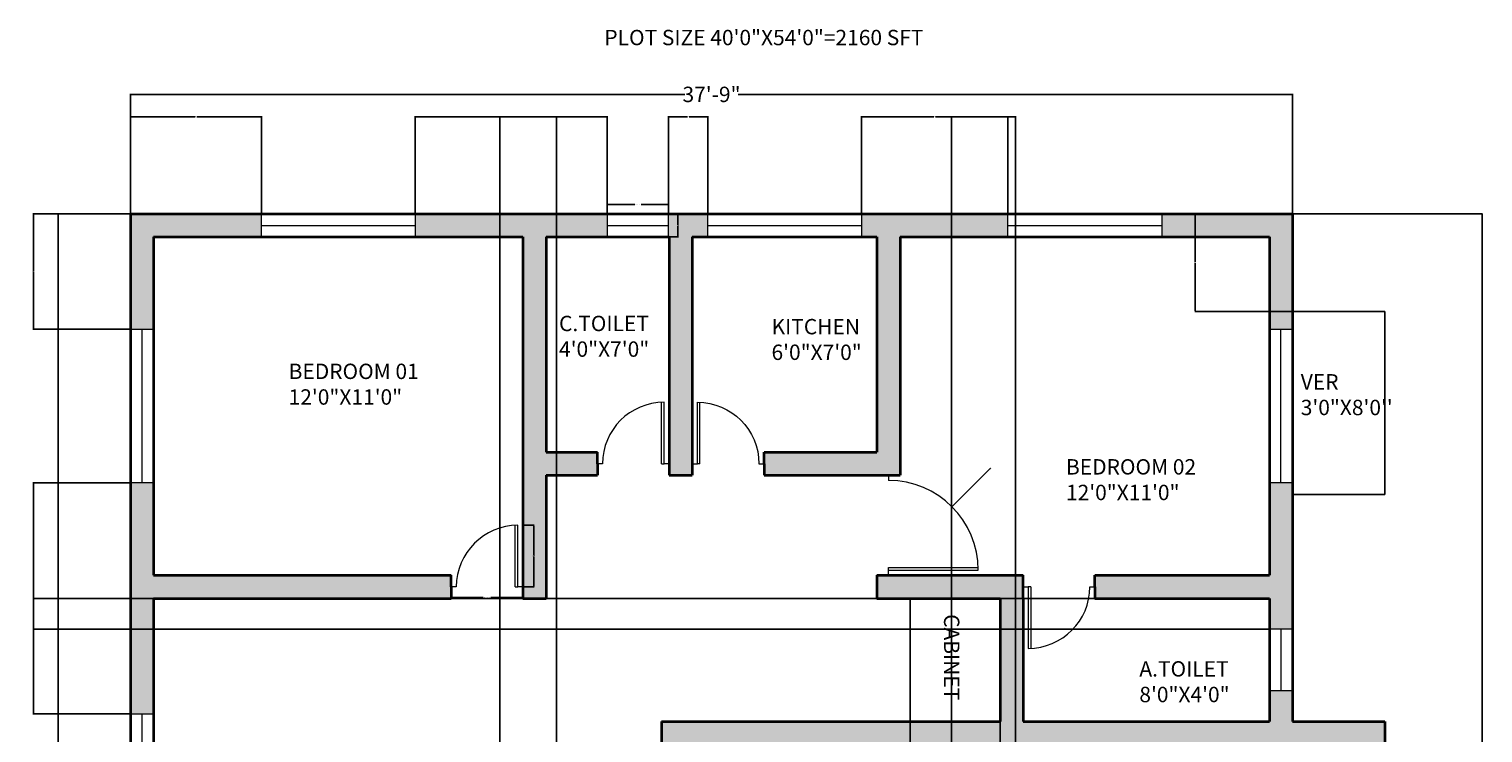
# Model space of a CAD drawing. Units: inches. Extents: x -17 to 550, y -704 to 87.
# Tile 2 of 2: x -17 to 550, y -187 to 87. Entities that reach past the tile are written whole.
import ezdxf

# ---------------------------------------------------------------- set-up
doc = ezdxf.new("R2010")
doc.units = ezdxf.units.IN
doc.header["$MEASUREMENT"] = 0
for name, color, linetype, lineweight in [('A-ANNO-DIMS', 2, 'Continuous', 18), ('A-ANNO-TEXT', 7, 'Continuous', 18), ('A-AREA-IDEN', 7, 'Continuous', 18), ('A-DOOR', 3, 'Continuous', 18), ('A-FLOR-CASE', 8, 'Continuous', 18), ('A-FLOR-OTLN', 7, 'Continuous', 25), ('A-GLAZ', 4, 'Continuous', 18), ('A-WALL', 7, 'Continuous', 35), ('A-WALL-PATT', 252, 'Continuous', 13)]:
    doc.layers.add(name, color=color, linetype=linetype, lineweight=lineweight)
doc.styles.get("Standard").update_dxf_attribs({"font": 'arial.ttf'})
doc.dimstyles.get("Standard").update_dxf_attribs({"dimtxt": 0.18, "dimasz": 0.18, "dimexe": 0.18, "dimexo": 0.0625, "dimgap": 0.09, "dimtad": 0, "dimtih": 1, "dimtoh": 1, "dimdec": 0, "dimzin": 0, "dimdsep": 46, "dimlunit": 3, "dimtxsty": 'Standard', "dimcen": 0.09, "dimadec": 0, "dimazin": 0, "dimtfac": 1, "dimtdec": 0, "dimtofl": 0, "dimtmove": 0, "dimatfit": 3, "dimfxl": 1, "dimtolj": 1, "dimtzin": 0, "dimarcsym": 0})

# ---------------------------------------------------------------- blocks, each defined once
blk = doc.blocks.new('*D1')
at = {"layer": 'A-ANNO-DIMS', "color": 0, "lineweight": -2, "transparency": 16777216}
for p, q in [((22.74, 15.39), (22.74, 62.1)), ((22.92, 61.92), (238.85, 61.92)), ((475.56, 61.92), (259.64, 61.92)), ((475.74, 15.39), (475.74, 62.1))]:
    blk.add_line(p, q, dxfattribs=at)
at = {"layer": 'A-ANNO-DIMS', "color": 0, "transparency": 16777216}
for points in [[(22.92, 61.95), (22.92, 61.89), (22.74, 61.92)], [(475.56, 61.95), (475.56, 61.89), (475.74, 61.92)]]:
    blk.add_solid(points, dxfattribs=at)
at = {"layer": 'Defpoints', "color": 0, "transparency": 16777216}
for p in [(475.74, 61.92), (22.74, 15.33), (475.74, 15.33)]:
    blk.add_point(p, dxfattribs=at)
at = {"layer": 'A-ANNO-DIMS', "color": 0, "transparency": 16777216, "insert": (249.24, 61.92), "char_height": 6, "attachment_point": 5}
blk.add_mtext('\\A1;37\'-9"', dxfattribs=at)
blk = doc.blocks.new('*D2')
at = {"layer": 'A-ANNO-DIMS', "color": 0, "lineweight": -2, "transparency": 16777216}
for p, q in [((22.68, 15.33), (-5.69, 15.33)), ((-5.51, 15.15), (-5.51, -322.02)), ((-5.51, -665.49), (-5.51, -328.33)), ((22.68, -665.67), (-5.69, -665.67))]:
    blk.add_line(p, q, dxfattribs=at)
at = {"layer": 'A-ANNO-DIMS', "color": 0, "transparency": 16777216}
for points in [[(-5.54, 15.15), (-5.48, 15.15), (-5.51, 15.33)], [(-5.54, -665.49), (-5.48, -665.49), (-5.51, -665.67)]]:
    blk.add_solid(points, dxfattribs=at)
at = {"layer": 'Defpoints', "color": 0, "transparency": 16777216}
for p in [(22.74, 15.33), (-5.51, -665.67), (22.74, -665.67)]:
    blk.add_point(p, dxfattribs=at)
at = {"layer": 'A-ANNO-DIMS', "color": 0, "transparency": 16777216, "insert": (-5.51, -325.17), "char_height": 6, "attachment_point": 5}
blk.add_mtext('\\A1;56\'-9"', dxfattribs=at)
blk = doc.blocks.new('WIN-60IN')
for p, q in [((0, 9), (60, 9)), ((0, 0), (0, 9)), ((60, 9), (60, 0)), ((0, 4.5), (60, 4.5)), ((60, 0), (0, 0))]:
    blk.add_line(p, q)
blk = doc.blocks.new('WIN-24IN')
for p, q in [((0, 24), (0, 0)), ((9, 24), (0, 24)), ((4.5, 24), (4.5, 0)), ((9, 0), (9, 24)), ((0, 0), (9, 0))]:
    blk.add_line(p, q)
blk = doc.blocks.new('DOOR-SWING-24IN')
for p, q in [((25, 0), (25, 24)), ((26, 0), (26, 24)), ((2, 0), (0, 0)), ((25, 0), (26, 0)), ((28, 0), (26, 0))]:
    blk.add_line(p, q)
blk.add_arc((26, 0), 24, 90, 180)
blk = doc.blocks.new('*D8')
at = {"layer": 'A-ANNO-DIMS', "color": 0, "lineweight": -2, "transparency": 16777216}
for p, q in [((147.74, -130.24), (147.74, -134.55)), ((175.74, -130.24), (175.74, -134.55)), ((147.92, -134.37), (160.23, -134.37)), ((175.56, -134.37), (163.25, -134.37))]:
    blk.add_line(p, q, dxfattribs=at)
at = {"layer": 'A-ANNO-DIMS', "color": 0, "transparency": 16777216}
for points in [[(147.92, -134.34), (147.92, -134.4), (147.74, -134.37)], [(175.56, -134.34), (175.56, -134.4), (175.74, -134.37)]]:
    blk.add_solid(points, dxfattribs=at)
at = {"layer": 'Defpoints', "color": 0, "transparency": 16777216}
for p in [(147.74, -130.17), (175.74, -130.17), (175.74, -134.37)]:
    blk.add_point(p, dxfattribs=at)
at = {"layer": 'A-ANNO-DIMS', "color": 0, "transparency": 16777216, "insert": (161.74, -134.37), "char_height": 0.18, "attachment_point": 5}
blk.add_mtext('\\A1;SWING DOOR 2\'-4" TYP.', dxfattribs=at)
blk = doc.blocks.new('*D9')
at = {"layer": 'A-ANNO-DIMS', "color": 0, "lineweight": -2, "transparency": 16777216}
for p, q in [((175.81, -106.17), (180.12, -106.17)), ((179.94, -106.35), (179.94, -117.99)), ((179.94, -129.99), (179.94, -118.36)), ((175.81, -130.17), (180.12, -130.17))]:
    blk.add_line(p, q, dxfattribs=at)
at = {"layer": 'A-ANNO-DIMS', "color": 0, "transparency": 16777216}
for points in [[(179.91, -106.35), (179.97, -106.35), (179.94, -106.17)], [(179.91, -129.99), (179.97, -129.99), (179.94, -130.17)]]:
    blk.add_solid(points, dxfattribs=at)
at = {"layer": 'Defpoints', "color": 0, "transparency": 16777216}
for p in [(175.74, -106.17), (179.94, -106.17), (175.74, -130.17)]:
    blk.add_point(p, dxfattribs=at)
at = {"layer": 'A-ANNO-DIMS', "color": 0, "transparency": 16777216, "insert": (179.94, -118.17), "char_height": 0.18, "attachment_point": 5}
blk.add_mtext('\\A1;2\'-0" TYP.', dxfattribs=at)
blk = doc.blocks.new('*D12')
at = {"layer": 'A-ANNO-DIMS', "color": 0, "lineweight": -2, "transparency": 16777216}
for p, q in [((208.53, 15.39), (208.53, 19.11)), ((208.71, 18.93), (219.31, 18.93)), ((232.35, 18.93), (221.76, 18.93)), ((232.53, 15.39), (232.53, 19.11))]:
    blk.add_line(p, q, dxfattribs=at)
at = {"layer": 'A-ANNO-DIMS', "color": 0, "transparency": 16777216}
for points in [[(208.71, 18.96), (208.71, 18.9), (208.53, 18.93)], [(232.35, 18.96), (232.35, 18.9), (232.53, 18.93)]]:
    blk.add_solid(points, dxfattribs=at)
at = {"layer": 'Defpoints', "color": 0, "transparency": 16777216}
for p in [(208.53, 18.93), (208.53, 15.33), (232.53, 15.33)]:
    blk.add_point(p, dxfattribs=at)
at = {"layer": 'A-ANNO-DIMS', "color": 0, "transparency": 16777216, "insert": (220.53, 18.93), "char_height": 0.18, "attachment_point": 5}
blk.add_mtext('\\A1;WINDOW 2\'-0" TYP.', dxfattribs=at)
blk = doc.blocks.new('*D13')
at = {"layer": 'A-ANNO-DIMS', "color": 0, "lineweight": -2, "transparency": 16777216}
for p, q in [((232.6, 15.33), (236.31, 15.33)), ((236.13, 15.15), (236.13, 11.01)), ((232.6, 6.33), (236.31, 6.33)), ((236.13, 6.51), (236.13, 10.64))]:
    blk.add_line(p, q, dxfattribs=at)
at = {"layer": 'A-ANNO-DIMS', "color": 0, "transparency": 16777216}
for points in [[(236.1, 15.15), (236.16, 15.15), (236.13, 15.33)], [(236.1, 6.51), (236.16, 6.51), (236.13, 6.33)]]:
    blk.add_solid(points, dxfattribs=at)
at = {"layer": 'Defpoints', "color": 0, "transparency": 16777216}
for p in [(232.53, 15.33), (236.13, 15.33), (232.53, 6.33)]:
    blk.add_point(p, dxfattribs=at)
at = {"layer": 'A-ANNO-DIMS', "color": 0, "transparency": 16777216, "insert": (236.13, 10.83), "char_height": 0.18, "attachment_point": 5}
blk.add_mtext('\\A1;0\'-9" TYP.', dxfattribs=at)
blk = doc.blocks.new('*D23')
at = {"layer": 'A-ANNO-DIMS', "color": 0, "lineweight": -2, "transparency": 16777216}
for p, q in [((22.74, 15.39), (22.74, 53.41)), ((22.92, 53.23), (47.91, 53.23)), ((73.56, 53.23), (48.58, 53.23)), ((73.74, 15.39), (73.74, 53.41))]:
    blk.add_line(p, q, dxfattribs=at)
at = {"layer": 'A-ANNO-DIMS', "color": 0, "transparency": 16777216}
for points in [[(22.92, 53.26), (22.92, 53.2), (22.74, 53.23)], [(73.56, 53.26), (73.56, 53.2), (73.74, 53.23)]]:
    blk.add_solid(points, dxfattribs=at)
at = {"layer": 'Defpoints', "color": 0, "transparency": 16777216}
for p in [(73.74, 53.23), (22.74, 15.33), (73.74, 15.33)]:
    blk.add_point(p, dxfattribs=at)
at = {"layer": 'A-ANNO-DIMS', "color": 0, "transparency": 16777216, "insert": (48.24, 53.23), "char_height": 0.18, "attachment_point": 5}
blk.add_mtext('\\A1;4\'-3"', dxfattribs=at)
blk = doc.blocks.new('*D24')
at = {"layer": 'A-ANNO-DIMS', "color": 0, "lineweight": -2, "transparency": 16777216}
for p, q in [((133.74, 15.39), (133.74, 53.41)), ((133.92, 53.23), (170.81, 53.23)), ((208.35, 53.23), (171.47, 53.23)), ((208.53, 15.39), (208.53, 53.41))]:
    blk.add_line(p, q, dxfattribs=at)
at = {"layer": 'A-ANNO-DIMS', "color": 0, "transparency": 16777216}
for points in [[(133.92, 53.26), (133.92, 53.2), (133.74, 53.23)], [(208.35, 53.26), (208.35, 53.2), (208.53, 53.23)]]:
    blk.add_solid(points, dxfattribs=at)
at = {"layer": 'Defpoints', "color": 0, "transparency": 16777216}
for p in [(208.53, 53.23), (133.74, 15.33), (208.53, 15.33)]:
    blk.add_point(p, dxfattribs=at)
at = {"layer": 'A-ANNO-DIMS', "color": 0, "transparency": 16777216, "insert": (171.14, 53.23), "char_height": 0.18, "attachment_point": 5}
blk.add_mtext('\\A1;6\'-3"', dxfattribs=at)
blk = doc.blocks.new('*D25')
at = {"layer": 'A-ANNO-DIMS', "color": 0, "lineweight": -2, "transparency": 16777216}
for p, q in [((232.53, 15.39), (232.53, 53.41)), ((232.71, 53.23), (239.82, 53.23)), ((247.56, 53.23), (240.46, 53.23)), ((247.74, 15.39), (247.74, 53.41))]:
    blk.add_line(p, q, dxfattribs=at)
at = {"layer": 'A-ANNO-DIMS', "color": 0, "transparency": 16777216}
for points in [[(232.71, 53.26), (232.71, 53.2), (232.53, 53.23)], [(247.56, 53.26), (247.56, 53.2), (247.74, 53.23)]]:
    blk.add_solid(points, dxfattribs=at)
at = {"layer": 'Defpoints', "color": 0, "transparency": 16777216}
for p in [(247.74, 53.23), (232.53, 15.33), (247.74, 15.33)]:
    blk.add_point(p, dxfattribs=at)
at = {"layer": 'A-ANNO-DIMS', "color": 0, "transparency": 16777216, "insert": (240.14, 53.23), "char_height": 0.18, "attachment_point": 5}
blk.add_mtext('\\A1;1\'-3"', dxfattribs=at)
blk = doc.blocks.new('*D26')
at = {"layer": 'A-ANNO-DIMS', "color": 0, "lineweight": -2, "transparency": 16777216}
for p, q in [((307.74, 15.39), (307.74, 53.41)), ((307.92, 53.23), (335.91, 53.23)), ((364.56, 53.23), (336.58, 53.23)), ((364.74, 15.39), (364.74, 53.41))]:
    blk.add_line(p, q, dxfattribs=at)
at = {"layer": 'A-ANNO-DIMS', "color": 0, "transparency": 16777216}
for points in [[(307.92, 53.26), (307.92, 53.2), (307.74, 53.23)], [(364.56, 53.26), (364.56, 53.2), (364.74, 53.23)]]:
    blk.add_solid(points, dxfattribs=at)
at = {"layer": 'Defpoints', "color": 0, "transparency": 16777216}
for p in [(364.74, 53.23), (307.74, 15.33), (364.74, 15.33)]:
    blk.add_point(p, dxfattribs=at)
at = {"layer": 'A-ANNO-DIMS', "color": 0, "transparency": 16777216, "insert": (336.24, 53.23), "char_height": 0.18, "attachment_point": 5}
blk.add_mtext('\\A1;4\'-9"', dxfattribs=at)
blk = doc.blocks.new('*D27')
at = {"layer": 'A-ANNO-DIMS', "color": 0, "lineweight": -2, "transparency": 16777216}
for p, q in [((22.68, 15.33), (-15.34, 15.33)), ((-15.16, 15.15), (-15.16, -6.99)), ((-15.16, -29.49), (-15.16, -7.36)), ((22.68, -29.67), (-15.34, -29.67))]:
    blk.add_line(p, q, dxfattribs=at)
at = {"layer": 'A-ANNO-DIMS', "color": 0, "transparency": 16777216}
for points in [[(-15.19, 15.15), (-15.13, 15.15), (-15.16, 15.33)], [(-15.19, -29.49), (-15.13, -29.49), (-15.16, -29.67)]]:
    blk.add_solid(points, dxfattribs=at)
at = {"layer": 'Defpoints', "color": 0, "transparency": 16777216}
for p in [(-15.16, 15.33), (22.74, 15.33), (22.74, -29.67)]:
    blk.add_point(p, dxfattribs=at)
at = {"layer": 'A-ANNO-DIMS', "color": 0, "transparency": 16777216, "insert": (-15.16, -7.17), "char_height": 0.18, "attachment_point": 5}
blk.add_mtext('\\A1;3\'-9"', dxfattribs=at)
blk = doc.blocks.new('*D28')
at = {"layer": 'A-ANNO-DIMS', "color": 0, "lineweight": -2, "transparency": 16777216}
for p, q in [((22.68, -89.67), (-15.34, -89.67)), ((-15.16, -89.85), (-15.16, -134.49)), ((-15.16, -179.49), (-15.16, -134.86)), ((22.68, -179.67), (-15.34, -179.67))]:
    blk.add_line(p, q, dxfattribs=at)
at = {"layer": 'A-ANNO-DIMS', "color": 0, "transparency": 16777216}
for points in [[(-15.19, -89.85), (-15.13, -89.85), (-15.16, -89.67)], [(-15.19, -179.49), (-15.13, -179.49), (-15.16, -179.67)]]:
    blk.add_solid(points, dxfattribs=at)
at = {"layer": 'Defpoints', "color": 0, "transparency": 16777216}
for p in [(-15.16, -89.67), (22.74, -89.67), (22.74, -179.67)]:
    blk.add_point(p, dxfattribs=at)
at = {"layer": 'A-ANNO-DIMS', "color": 0, "transparency": 16777216, "insert": (-15.16, -134.67), "char_height": 0.18, "attachment_point": 5}
blk.add_mtext('\\A1;7\'-6"', dxfattribs=at)
blk = doc.blocks.new('*D32')
at = {"layer": 'A-ANNO-DIMS', "color": 0, "lineweight": -2, "transparency": 16777216}
for p, q in [((326.67, -134.74), (326.67, -703.75)), ((361.74, -134.74), (361.74, -703.75)), ((326.85, -703.57), (343.81, -703.57)), ((361.56, -703.57), (344.61, -703.57))]:
    blk.add_line(p, q, dxfattribs=at)
at = {"layer": 'A-ANNO-DIMS', "color": 0, "transparency": 16777216}
for points in [[(326.85, -703.54), (326.85, -703.6), (326.67, -703.57)], [(361.56, -703.54), (361.56, -703.6), (361.74, -703.57)]]:
    blk.add_solid(points, dxfattribs=at)
at = {"layer": 'Defpoints', "color": 0, "transparency": 16777216}
for p in [(326.67, -134.67), (361.74, -134.67), (361.74, -703.57)]:
    blk.add_point(p, dxfattribs=at)
at = {"layer": 'A-ANNO-DIMS', "color": 0, "transparency": 16777216, "insert": (344.21, -703.57), "char_height": 0.18, "attachment_point": 5}
blk.add_mtext('\\A1;2\'-11"', dxfattribs=at)
blk = doc.blocks.new('*D33')
at = {"layer": 'A-ANNO-DIMS', "color": 0, "lineweight": -2, "transparency": 16777216}
for p, q in [((166.74, -632.61), (166.74, 53.41)), ((166.92, 53.23), (177.41, 53.23)), ((188.68, 53.23), (178.19, 53.23)), ((188.86, -632.61), (188.86, 53.41))]:
    blk.add_line(p, q, dxfattribs=at)
at = {"layer": 'A-ANNO-DIMS', "color": 0, "transparency": 16777216}
for points in [[(166.92, 53.26), (166.92, 53.2), (166.74, 53.23)], [(188.68, 53.26), (188.68, 53.2), (188.86, 53.23)]]:
    blk.add_solid(points, dxfattribs=at)
at = {"layer": 'Defpoints', "color": 0, "transparency": 16777216}
for p in [(188.86, 53.23), (166.74, -632.67), (188.86, -632.67)]:
    blk.add_point(p, dxfattribs=at)
at = {"layer": 'A-ANNO-DIMS', "color": 0, "transparency": 16777216, "insert": (177.8, 53.23), "char_height": 0.18, "attachment_point": 5}
blk.add_mtext('\\A1;1\'-10"', dxfattribs=at)
blk = doc.blocks.new('*D34')
at = {"layer": 'A-ANNO-DIMS', "color": 0, "lineweight": -2, "transparency": 16777216}
for p, q in [((342.82, -632.61), (342.82, 53.41)), ((343, 53.23), (354.95, 53.23)), ((367.56, 53.23), (355.61, 53.23)), ((367.74, -632.61), (367.74, 53.41))]:
    blk.add_line(p, q, dxfattribs=at)
at = {"layer": 'A-ANNO-DIMS', "color": 0, "transparency": 16777216}
for points in [[(343, 53.26), (343, 53.2), (342.82, 53.23)], [(367.56, 53.26), (367.56, 53.2), (367.74, 53.23)]]:
    blk.add_solid(points, dxfattribs=at)
at = {"layer": 'Defpoints', "color": 0, "transparency": 16777216}
for p in [(367.74, 53.23), (342.82, -632.67), (367.74, -632.67)]:
    blk.add_point(p, dxfattribs=at)
at = {"layer": 'A-ANNO-DIMS', "color": 0, "transparency": 16777216, "insert": (355.28, 53.23), "char_height": 0.18, "attachment_point": 5}
blk.add_mtext('\\A1;2\'-1"', dxfattribs=at)
blk = doc.blocks.new('*D39')
at = {"layer": 'A-ANNO-DIMS', "color": 0, "lineweight": -2, "transparency": 16777216}
for p, q in [((466.68, -134.67), (-15.34, -134.67)), ((-15.16, -134.85), (-15.16, -140.49)), ((-15.16, -146.49), (-15.16, -140.86)), ((466.68, -146.67), (-15.34, -146.67))]:
    blk.add_line(p, q, dxfattribs=at)
at = {"layer": 'A-ANNO-DIMS', "color": 0, "transparency": 16777216}
for points in [[(-15.19, -134.85), (-15.13, -134.85), (-15.16, -134.67)], [(-15.19, -146.49), (-15.13, -146.49), (-15.16, -146.67)]]:
    blk.add_solid(points, dxfattribs=at)
at = {"layer": 'Defpoints', "color": 0, "transparency": 16777216}
for p in [(466.74, -134.67), (-15.16, -146.67), (466.74, -146.67)]:
    blk.add_point(p, dxfattribs=at)
at = {"layer": 'A-ANNO-DIMS', "color": 0, "transparency": 16777216, "insert": (-15.16, -140.67), "char_height": 0.18, "attachment_point": 5}
blk.add_mtext('\\A1;1\'-0"', dxfattribs=at)
blk = doc.blocks.new('*D40')
at = {"layer": 'A-ANNO-DIMS', "color": 0, "lineweight": -2, "transparency": 16777216}
for p, q in [((475.68, 15.33), (437.66, 15.33)), ((437.84, 15.15), (437.84, -3.51)), ((437.84, -22.53), (437.84, -3.87)), ((475.68, -22.71), (437.66, -22.71))]:
    blk.add_line(p, q, dxfattribs=at)
at = {"layer": 'A-ANNO-DIMS', "color": 0, "transparency": 16777216}
for points in [[(437.81, 15.15), (437.87, 15.15), (437.84, 15.33)], [(437.81, -22.53), (437.87, -22.53), (437.84, -22.71)]]:
    blk.add_solid(points, dxfattribs=at)
at = {"layer": 'Defpoints', "color": 0, "transparency": 16777216}
for p in [(437.84, 15.33), (475.74, 15.33), (475.74, -22.71)]:
    blk.add_point(p, dxfattribs=at)
at = {"layer": 'A-ANNO-DIMS', "color": 0, "transparency": 16777216, "insert": (437.84, -3.69), "char_height": 0.18, "attachment_point": 5}
blk.add_mtext('\\A1;3\'-2"', dxfattribs=at)
blk = doc.blocks.new('*D41')
at = {"layer": 'A-ANNO-DIMS', "color": 0, "lineweight": -2, "transparency": 16777216}
for p, q in [((475.81, 15.33), (549.82, 15.33)), ((549.64, 15.15), (549.64, -324.99)), ((549.64, -665.49), (549.64, -325.36)), ((511.81, -665.67), (549.82, -665.67))]:
    blk.add_line(p, q, dxfattribs=at)
at = {"layer": 'A-ANNO-DIMS', "color": 0, "transparency": 16777216}
for points in [[(549.61, 15.15), (549.67, 15.15), (549.64, 15.33)], [(549.61, -665.49), (549.67, -665.49), (549.64, -665.67)]]:
    blk.add_solid(points, dxfattribs=at)
at = {"layer": 'Defpoints', "color": 0, "transparency": 16777216}
for p in [(475.74, 15.33), (549.64, 15.33), (511.74, -665.67)]:
    blk.add_point(p, dxfattribs=at)
at = {"layer": 'A-ANNO-DIMS', "color": 0, "transparency": 16777216, "insert": (549.64, -325.17), "char_height": 0.18, "attachment_point": 5}
blk.add_mtext('\\A1;56\'-9"', dxfattribs=at)
blk = doc.blocks.new('*D42')
at = {"layer": 'A-ANNO-DIMS', "color": 0, "lineweight": -2, "transparency": 16777216}
for p, q in [((357.84, -84.08), (343.12, -98.8)), ((358.02, -84.08), (357.84, -84.08)), ((318.15, -123.67), (318.33, -123.67)), ((318.24, -123.76), (318.24, -123.58))]:
    blk.add_line(p, q, dxfattribs=at)
at = {"layer": 'A-ANNO-DIMS', "color": 0, "transparency": 16777216}
blk.add_solid([(343.1, -98.78), (343.14, -98.82), (342.99, -98.93)], dxfattribs=at)
at = {"layer": 'Defpoints', "color": 0, "transparency": 16777216}
for p in [(342.99, -98.93), (318.24, -123.67)]:
    blk.add_point(p, dxfattribs=at)
at = {"layer": 'A-ANNO-DIMS', "color": 0, "transparency": 16777216, "insert": (358.51, -84.08), "char_height": 0.18, "attachment_point": 5}
blk.add_mtext('\\A1;R2\'-11"', dxfattribs=at)

msp = doc.modelspace()

# ---------------------------------------------------------------- hatches: boundary and pattern name
at = {"layer": 'A-WALL-PATT'}
h = msp.add_hatch(color=256, dxfattribs=at)
h.dxf.hatch_style = 1
h.paths.add_polyline_path([(322.74, 6.33), (364.74, 6.33), (364.74, 15.33), (307.74, 15.33), (307.74, 6.33), (313.74, 6.33), (313.74, -77.67), (269.74, -77.67), (269.74, -82.17), (269.74, -86.67), (322.74, -86.67)])
h.paths.add_polyline_path([(475.74, 15.33), (424.74, 15.33), (424.74, 6.33), (466.74, 6.33), (466.74, -29.67), (475.74, -29.67)])
h.paths.add_polyline_path([(475.74, -89.67), (466.74, -89.67), (466.74, -125.67), (398.74, -125.67), (398.74, -130.17), (398.74, -134.67), (466.74, -134.67), (466.74, -146.67), (475.74, -146.67)])
h.paths.add_polyline_path([(511.74, -182.67), (475.74, -182.67), (475.74, -170.67), (466.74, -170.67), (466.74, -182.67), (370.74, -182.67), (370.74, -134.67), (370.74, -125.67), (313.74, -125.67), (313.74, -134.67), (361.74, -134.67), (361.74, -182.67), (229.74, -182.67), (229.74, -194.67), (238.74, -194.67), (238.74, -191.67), (502.74, -191.67), (502.74, -208.17), (511.74, -208.17)])
h.paths.add_polyline_path([(184.74, -86.67), (204.74, -86.67), (204.74, -82.17), (204.74, -77.67), (184.74, -77.67), (184.74, 6.33), (208.53, 6.33), (208.53, 15.33), (133.74, 15.33), (133.74, 6.33), (175.74, 6.33), (175.74, -134.67), (184.74, -134.67)])
h.paths.add_polyline_path([(241.74, 6.33), (247.74, 6.33), (247.74, 15.33), (232.53, 15.33), (232.53, 6.33), (232.74, 6.33), (232.74, -86.67), (241.74, -86.67)])
h.paths.add_polyline_path([(147.74, -125.67), (31.74, -125.67), (31.74, -89.67), (22.74, -89.67), (22.74, -179.67), (31.74, -179.67), (31.74, -134.67), (147.74, -134.67), (147.74, -130.17)])
h.paths.add_polyline_path([(31.74, 6.33), (73.74, 6.33), (73.74, 15.33), (22.74, 15.33), (22.74, -29.67), (31.74, -29.67)])
h.paths.add_polyline_path([(238.74, -284.67), (238.74, -222.67), (234.24, -222.67), (229.74, -222.67), (229.74, -284.67), (31.74, -284.67), (31.74, -239.67), (22.74, -239.67), (22.74, -323.67), (31.74, -323.67), (31.74, -293.67), (157.74, -293.67), (157.74, -422.67), (166.74, -422.67), (166.74, -293.67), (238.74, -293.67)])
h.paths.add_polyline_path([(511.74, -268.17), (502.74, -268.17), (502.74, -284.67), (370.74, -284.67), (361.74, -284.67), (295.74, -284.67), (295.74, -289.17), (295.74, -293.67), (367.74, -293.67), (367.74, -422.67), (376.74, -422.67), (376.74, -413.67), (376.74, -293.67), (502.74, -293.67), (502.74, -323.67), (511.74, -323.67)])
h.paths.add_polyline_path([(511.74, -383.67), (502.74, -383.67), (502.74, -413.67), (404.74, -413.67), (404.74, -418.17), (404.74, -422.67), (502.74, -422.67), (502.74, -436.82), (511.74, -436.82)])
h.paths.add_polyline_path([(424.74, -422.67), (415.74, -422.67), (415.74, -448.67), (420.24, -448.67), (424.74, -448.67)])
h.paths.add_polyline_path([(511.74, -460.82), (502.74, -460.82), (502.74, -476.67), (376.74, -476.67), (367.74, -476.67), (367.74, -485.67), (376.74, -485.67), (502.74, -485.67), (502.74, -512.17), (511.74, -512.17)])
h.paths.add_polyline_path([(376.74, -513.67), (372.24, -513.67), (367.74, -513.67), (367.74, -527.67), (299.74, -527.67), (299.74, -532.17), (299.74, -536.67), (367.74, -536.67), (367.74, -632.67), (342.82, -632.67), (342.82, -641.67), (367.74, -641.67), (367.74, -665.67), (376.74, -665.67), (378.02, -665.67), (378.02, -656.67), (376.74, -656.67), (376.74, -614.67)])
h.paths.add_polyline_path([(511.74, -572.17), (502.74, -572.17), (502.74, -605.67), (511.74, -605.67)])
h.paths.add_polyline_path([(451.74, -605.67), (442.74, -605.67), (442.74, -656.67), (402.02, -656.67), (402.02, -665.67), (451.74, -665.67)])
h.paths.add_polyline_path([(414.74, -605.67), (376.74, -605.67), (376.74, -614.67), (414.74, -614.67), (414.74, -610.17)])
h.paths.add_polyline_path([(282.82, -632.67), (271.74, -632.67), (271.74, -293.67), (271.74, -284.67), (262.74, -284.67), (262.74, -293.67), (262.74, -632.67), (248.86, -632.67), (248.86, -641.67), (282.82, -641.67)])
h.paths.add_polyline_path([(166.74, -536.67), (234.74, -536.67), (234.74, -532.17), (234.74, -527.67), (166.74, -527.67), (166.74, -513.67), (162.24, -513.67), (157.74, -513.67), (157.74, -605.67), (119.74, -605.67), (119.74, -610.17), (119.74, -614.67), (157.74, -614.67), (157.74, -656.67), (157.43, -665.67), (166.74, -665.67)])
h.paths.add_polyline_path([(188.86, -632.67), (166.74, -632.67), (166.74, -641.67), (188.86, -641.67)], flags=17)
h.paths.add_polyline_path([(133.43, -656.67), (91.74, -656.67), (91.74, -605.67), (82.74, -605.67), (82.74, -665.67), (133.43, -665.67)])
h.paths.add_polyline_path([(31.74, -575.67), (22.74, -575.67), (22.74, -605.67), (31.74, -605.67)])
h.paths.add_polyline_path([(166.74, -476.67), (129.74, -476.67), (31.74, -476.67), (31.74, -461.67), (22.74, -461.67), (22.74, -515.67), (31.74, -515.67), (31.74, -485.67), (157.74, -485.67), (166.74, -485.67)])
h.paths.add_polyline_path([(129.74, -413.67), (31.74, -413.67), (31.74, -383.67), (22.74, -383.67), (22.74, -437.67), (31.74, -437.67), (31.74, -422.67), (109.74, -422.67), (109.74, -448.67), (114.24, -448.67), (118.74, -448.67), (118.74, -422.67), (129.74, -422.67), (129.74, -418.17)])

# ---------------------------------------------------------------- linework, layer by layer
at = {"layer": 'A-DOOR'}
for p, q in [((318.24, -86.67), (318.24, -88.67)), ((318.24, -122.67), (353.24, -122.67)), ((318.24, -123.67), (318.24, -122.67)), ((318.24, -125.67), (318.24, -123.67)), ((318.24, -123.67), (353.24, -123.67))]:
    msp.add_line(p, q, dxfattribs=at)
msp.add_arc((318.24, -123.67), 35, 0, 90, dxfattribs=at)
at = {"layer": 'A-FLOR-CASE'}
msp.add_line((326.67, -134.67), (326.67, -182.67), dxfattribs=at)
at = {"layer": 'A-FLOR-OTLN'}
for p, q in [((511.74, -22.71), (475.74, -22.71)), ((511.74, -22.71), (511.74, -94.13)), ((511.74, -94.13), (475.74, -94.13))]:
    msp.add_line(p, q, dxfattribs=at)
at = {"layer": 'A-WALL'}
for p, q in [((22.74, 15.33), (22.74, -665.67)), ((22.74, 15.33), (475.74, 15.33)), ((475.74, 15.33), (475.74, -182.67)), ((31.74, 6.33), (31.74, -125.67)), ((31.74, 6.33), (175.74, 6.33)), ((175.74, 6.33), (175.74, -134.67)), ((184.74, 6.33), (184.74, -77.67)), ((184.74, 6.33), (232.74, 6.33)), ((232.74, 6.33), (232.74, -86.67)), ((241.74, 6.33), (241.74, -86.67)), ((241.74, 6.33), (313.74, 6.33)), ((313.74, 6.33), (313.74, -77.67)), ((322.74, 6.33), (322.74, -86.67)), ((322.74, 6.33), (466.74, 6.33)), ((466.74, 6.33), (466.74, -125.67)), ((184.74, -77.67), (204.74, -77.67)), ((204.74, -82.17), (204.74, -77.67)), ((269.74, -77.67), (313.74, -77.67)), ((269.74, -82.17), (269.74, -77.67)), ((204.74, -82.17), (204.74, -86.67)), ((269.74, -82.17), (269.74, -86.67)), ((184.74, -86.67), (204.74, -86.67)), ((184.74, -86.67), (184.74, -134.67)), ((232.74, -86.67), (241.74, -86.67)), ((269.74, -86.67), (322.74, -86.67)), ((31.74, -125.67), (147.74, -125.67)), ((147.74, -130.17), (147.74, -125.67)), ((147.74, -130.17), (147.74, -134.67)), ((313.74, -125.67), (370.74, -125.67)), ((313.74, -125.67), (313.74, -134.67)), ((370.74, -134.67), (370.74, -125.67)), ((398.74, -130.17), (398.74, -125.67)), ((398.74, -125.67), (466.74, -125.67)), ((398.74, -130.17), (398.74, -134.67)), ((31.74, -134.67), (147.74, -134.67)), ((31.74, -134.67), (31.74, -284.67)), ((175.74, -134.67), (184.74, -134.67)), ((313.74, -134.67), (361.74, -134.67)), ((361.74, -134.67), (361.74, -182.67)), ((370.74, -134.67), (370.74, -182.67)), ((398.74, -134.67), (466.74, -134.67)), ((466.74, -134.67), (466.74, -182.67)), ((229.74, -182.67), (361.74, -182.67)), ((229.74, -182.67), (229.74, -194.67)), ((370.74, -182.67), (466.74, -182.67)), ((475.74, -182.67), (475.74, -182.67)), ((475.74, -182.67), (511.74, -182.67)), ((511.74, -182.67), (511.74, -641.67))]:
    msp.add_line(p, q, dxfattribs=at)

# ---------------------------------------------------------------- block references
at = {"layer": 'A-DOOR'}
for p in [(204.74, -82.17), (147.74, -130.17)]:
    msp.add_blockref('DOOR-SWING-24IN', p, dxfattribs=at)
at = {"layer": 'A-DOOR', "extrusion": (0, 0, -1), "zscale": -1}
msp.add_blockref('DOOR-SWING-24IN', (-269.74, -82.17), dxfattribs=at)
at = {"layer": 'A-DOOR', "rotation": 180}
msp.add_blockref('DOOR-SWING-24IN', (398.74, -130.17), dxfattribs=at)
at = {"layer": 'A-GLAZ'}
for name, p in [('WIN-60IN', (73.74, 6.33)), ('WIN-60IN', (247.74, 6.33)), ('WIN-60IN', (364.74, 6.33)), ('WIN-24IN', (466.74, -170.67))]:
    msp.add_blockref(name, p, dxfattribs=at)
for name, p, rotation in [('WIN-24IN', (232.53, 6.33), 89.99999999999952), ('WIN-60IN', (31.74, -89.67), 90.00000000000003), ('WIN-60IN', (475.74, -89.67), 90.00000000000003), ('WIN-60IN', (31.74, -239.67), 90.00000000000003)]:
    msp.add_blockref(name, p, dxfattribs=dict(at, rotation=rotation))

# ---------------------------------------------------------------- texts
at = {"layer": 'A-ANNO-TEXT', "insert": (207.45, 87.1), "char_height": 6, "attachment_point": 1}
msp.add_mtext('PLOT SIZE 40\'0"X54\'0"=2160 SFT', dxfattribs=at)
at = {"layer": 'A-ANNO-TEXT', "insert": (345.87, -140.82), "char_height": 6, "attachment_point": 1, "rotation": 270}
msp.add_mtext('CABINET', dxfattribs=at)
at = {"layer": 'A-AREA-IDEN', "char_height": 6, "attachment_point": 1}
for s, insert in [('C.TOILET\\P4\'0"X7\'0"', (189.78, -24.44)), ('KITCHEN\\P6\'0"X7\'0"', (272.63, -25.68)), ('BEDROOM 01\\P12\'0"X11\'0"', (84.36, -43.12)), ('VER\\P3\'0"X8\'0\'\'', (478.96, -47.21)), ('BEDROOM 02\\P12\'0"X11\'0"', (387.43, -80.37)), ('A.TOILET\\P8\'0"X4\'0"', (416.04, -159.18))]:
    msp.add_mtext(s, dxfattribs=dict(at, insert=insert))

# ---------------------------------------------------------------- dimensions: what is measured, and where the dimension line sits
at = {"layer": 'A-ANNO-DIMS'}
for base, p1, p2, override, picture, middle in [((475.74, 61.92), (22.74, 15.33), (475.74, 15.33), {"dimtxt": 6, "dimclrd": 0, "dimclre": 0, "dimclrt": 0}, '*D1', (249.24, 61.92)), ((73.74, 53.23), (22.74, 15.33), (73.74, 15.33), {"dimdec": 1, "dimlfac": 1, "dimrnd": 0, "dimzin": 1, "dimdsep": 46, "dimlunit": 4, "dimfrac": 2}, '*D23', (48.24, 53.23)), ((208.53, 53.23), (133.74, 15.33), (208.53, 15.33), {"dimdec": 1, "dimlfac": 1, "dimrnd": 0, "dimzin": 1, "dimdsep": 46, "dimlunit": 4, "dimfrac": 2}, '*D24', (171.14, 53.23)), ((188.86, 53.23), (166.74, -632.67), (188.86, -632.67), {"dimdec": 1, "dimlfac": 1, "dimrnd": 0, "dimzin": 1, "dimdsep": 46, "dimlunit": 4, "dimfrac": 2}, '*D33', (177.8, 53.23)), ((247.74, 53.23), (232.53, 15.33), (247.74, 15.33), {"dimdec": 1, "dimlfac": 1, "dimrnd": 0, "dimzin": 1, "dimdsep": 46, "dimlunit": 4, "dimfrac": 2}, '*D25', (240.14, 53.23)), ((364.74, 53.23), (307.74, 15.33), (364.74, 15.33), {"dimdec": 1, "dimlfac": 1, "dimrnd": 0, "dimzin": 1, "dimdsep": 46, "dimlunit": 4, "dimfrac": 2}, '*D26', (336.24, 53.23)), ((367.74, 53.23), (342.82, -632.67), (367.74, -632.67), {"dimdec": 1, "dimlfac": 1, "dimrnd": 0, "dimzin": 1, "dimdsep": 46, "dimlunit": 4, "dimfrac": 2}, '*D34', (355.28, 53.23)), ((361.74, -703.57), (326.67, -134.67), (361.74, -134.67), {"dimdec": 1, "dimlfac": 1, "dimrnd": 0, "dimzin": 1, "dimdsep": 46, "dimlunit": 4, "dimfrac": 2}, '*D32', (344.21, -703.57))]:
    dim = msp.add_linear_dim(base=base, p1=p1, p2=p2, dimstyle='Standard', override=override, dxfattribs=at)
    dim.commit()
    dim.dimension.update_dxf_attribs({"geometry": picture, "text_midpoint": middle})
for base, p1, p2, angle, text, picture, middle in [((208.53, 18.93), (232.53, 15.33), (208.53, 15.33), 180, 'WINDOW <> TYP.', '*D12', (220.53, 18.93)), ((236.13, 15.33), (232.53, 6.33), (232.53, 15.33), 90, '<> TYP.', '*D13', (236.13, 10.83)), ((179.94, -106.17), (175.74, -130.17), (175.74, -106.17), 90, '<> TYP.', '*D9', (179.94, -118.17))]:
    dim = msp.add_linear_dim(base=base, p1=p1, p2=p2, angle=angle, text=text, dimstyle='Standard', override={"dimdec": 1, "dimlfac": 1, "dimrnd": 0, "dimzin": 1, "dimdsep": 46, "dimlunit": 4, "dimfrac": 2}, dxfattribs=at)
    dim.commit()
    dim.dimension.update_dxf_attribs({"geometry": picture, "text_midpoint": middle})
for base, p1, p2, override, picture, middle in [((-5.51, -665.67), (22.74, 15.33), (22.74, -665.67), {"dimtxt": 6, "dimclrd": 0, "dimclre": 0, "dimclrt": 0}, '*D2', (-5.51, -325.17)), ((-15.16, 15.33), (22.74, -29.67), (22.74, 15.33), {"dimdec": 1, "dimlfac": 1, "dimrnd": 0, "dimzin": 1, "dimdsep": 46, "dimlunit": 4, "dimfrac": 2}, '*D27', (-15.16, -7.17)), ((437.84, 15.33), (475.74, -22.71), (475.74, 15.33), {"dimdec": 1, "dimlfac": 1, "dimrnd": 0, "dimzin": 1, "dimdsep": 46, "dimlunit": 4, "dimfrac": 2}, '*D40', (437.84, -3.69)), ((549.64, 15.33), (511.74, -665.67), (475.74, 15.33), {"dimdec": 1, "dimlfac": 1, "dimrnd": 0, "dimzin": 1, "dimdsep": 46, "dimlunit": 4, "dimfrac": 2}, '*D41', (549.64, -325.17)), ((-15.16, -89.67), (22.74, -179.67), (22.74, -89.67), {"dimdec": 1, "dimlfac": 1, "dimrnd": 0, "dimzin": 1, "dimdsep": 46, "dimlunit": 4, "dimfrac": 2}, '*D28', (-15.16, -134.67)), ((-15.16, -146.67), (466.74, -134.67), (466.74, -146.67), {"dimdec": 1, "dimlfac": 1, "dimrnd": 0, "dimzin": 1, "dimdsep": 46, "dimlunit": 4, "dimfrac": 2}, '*D39', (-15.16, -140.67))]:
    dim = msp.add_linear_dim(base=base, p1=p1, p2=p2, angle=90, dimstyle='Standard', override=override, dxfattribs=at)
    dim.commit()
    dim.dimension.update_dxf_attribs({"geometry": picture, "text_midpoint": middle})
dim = msp.add_radius_dim(center=(318.24, -123.67), mpoint=(342.99, -98.93), dimstyle='Standard', override={"dimdec": 1, "dimlfac": 1, "dimrnd": 0, "dimzin": 1, "dimdsep": 46, "dimlunit": 4, "dimfrac": 2}, dxfattribs=at)
dim.commit()
dim.dimension.update_dxf_attribs({"geometry": '*D42', "text_midpoint": (358.51, -84.08), "dimtype": 164})
dim = msp.add_linear_dim(base=(175.74, -134.37), p1=(147.74, -130.17), p2=(175.74, -130.17), text='SWING DOOR <> TYP.', dimstyle='Standard', override={"dimdec": 1, "dimlfac": 1, "dimrnd": 0, "dimzin": 1, "dimdsep": 46, "dimlunit": 4, "dimfrac": 2}, dxfattribs=at)
dim.commit()
dim.dimension.update_dxf_attribs({"geometry": '*D8', "text_midpoint": (161.74, -134.37)})

doc.saveas('drawing.dxf')
